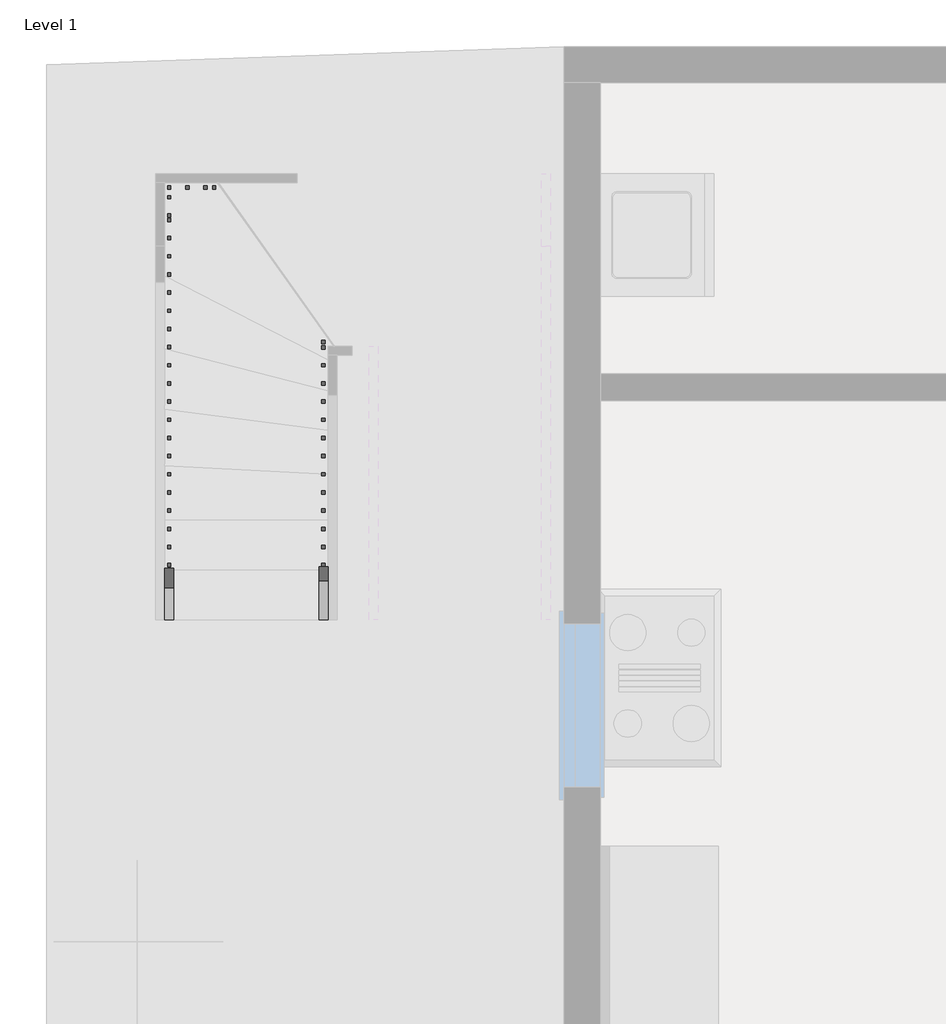
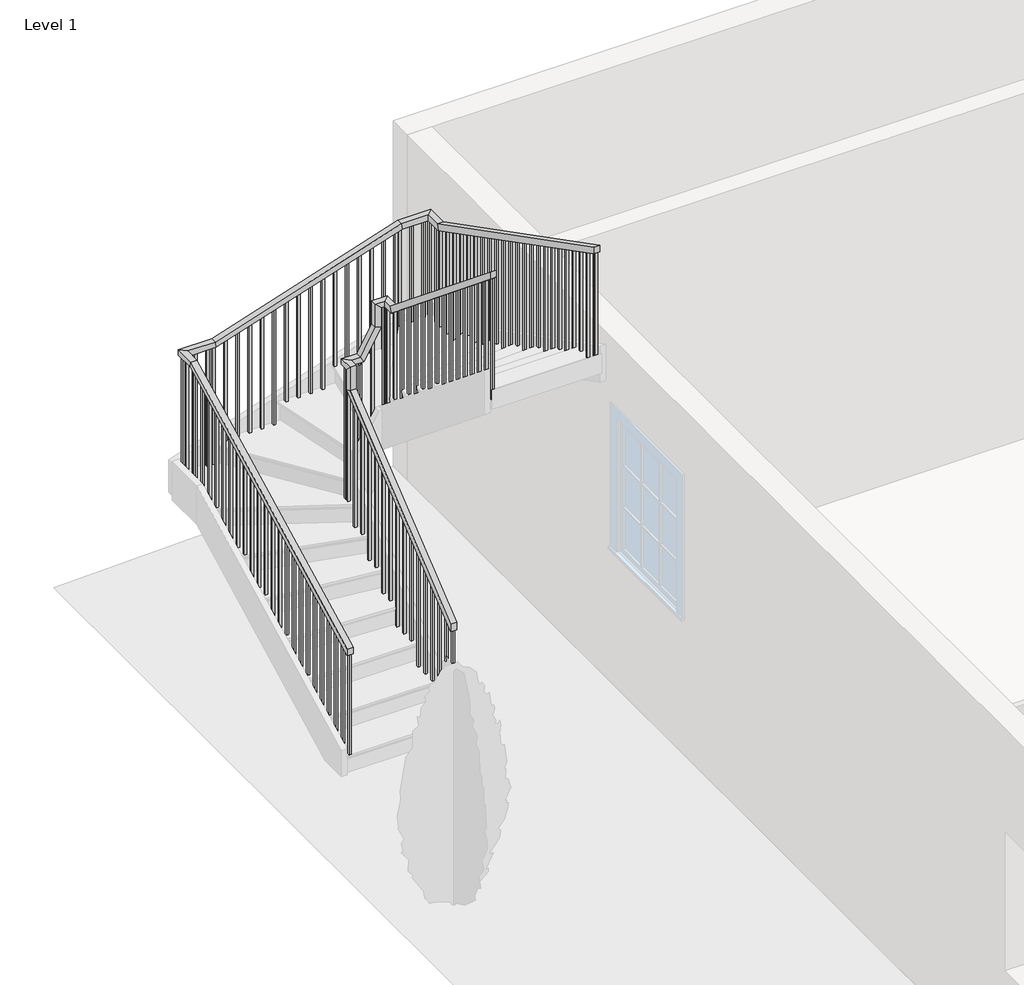
# One storey, part 2 of 3: 2 railings.
"""IFC4 building model written with IfcOpenShell, lengths in millimetres."""

from ifc_helpers import new_model, si_unit, frame, origin, place, context, project, spatial, polyline, outline, extrude, faceted_brep, element, save

model = new_model("IFC4")

# Units and contexts
model_context = context("Model", 3, world=origin())
ifc_project = project(units=[si_unit("LENGTHUNIT", "METRE", prefix="MILLI")], contexts=[model_context])

# Site, building, storey
site = spatial("IfcSite", under=ifc_project)
building = spatial("IfcBuilding", under=site)
storey = spatial("IfcBuildingStorey", under=building, Name="Level 1", Elevation=0.0)

# Railings
placement = place(None, origin())
element("IfcRailing", 1, ObjectType="Handrail - Rectangular", at=placement, inside=storey, context=model_context, shape_type="SolidModel", body=[
    faceted_brep([(-12458.9357228, 11608.7303252, 1025.2529681), (-12458.9357228, 11608.7303252, 959.7067088), (-12408.1357228, 11608.7303252, 959.7067088), (-12408.1357228, 11608.7303252, 1025.2529681), (-12458.9357228, 13060.2620171, 2208.7848338), (-12458.9357228, 13111.0620171, 2184.659247), (-12408.1357228, 13111.0620171, 2184.659247), (-12408.1357228, 13060.2620171, 2208.7848338), (-12458.9357228, 13060.2620171, 2414.6281882), (-12458.9357228, 13111.0620171, 2363.8281882), (-12408.1357228, 13111.0620171, 2363.8281882), (-12408.1357228, 13060.2620171, 2414.6281882), (-12458.9357228, 13187.2620171, 2414.6281882), (-12458.9357228, 13187.2620171, 2363.8281882), (-12408.1357228, 13136.4620171, 2363.8281882), (-12408.1357228, 13136.4620171, 2414.6281882), (-12331.9357228, 13187.2620171, 2414.6281882), (-12302.8143889, 13187.2620171, 2363.8281882), (-12302.8143889, 13136.4620171, 2363.8281882), (-12331.9357228, 13136.4620171, 2414.6281882), (-12204.9357228, 13187.2620171, 2631.5051451), (-12154.1357228, 13187.2620171, 2617.7256424), (-12154.1357228, 13136.4620171, 2617.7256424), (-12204.9357228, 13136.4620171, 2631.5051451), (-12204.9357228, 13187.2620171, 2837.3484995), (-12154.1357228, 13187.2620171, 2786.5484995), (-12154.1357228, 13136.4620171, 2786.5484995), (-12204.9357228, 13136.4620171, 2837.3484995), (-12077.9357228, 13187.2620171, 2837.3484995), (-12077.9357228, 13187.2620171, 2786.5484995), (-12128.7357228, 13136.4620171, 2786.5484995), (-12128.7357228, 13136.4620171, 2837.3484995), (-12077.9357228, 13060.2620171, 2837.3484995), (-12077.9357228, 13042.176604, 2786.5484995), (-12128.7357228, 13042.176604, 2786.5484995), (-12128.7357228, 13060.2620171, 2837.3484995), (-12077.9357228, 11608.7303252, 4020.8803652), (-12128.7357228, 11608.7303252, 4020.8803652), (-12128.7357228, 11608.7303252, 3955.3341059), (-12077.9357228, 11608.7303252, 3955.3341059)], [[[0, 1, 2, 3]], [[1, 0, 4, 5]], [[2, 1, 5, 6]], [[3, 2, 6, 7]], [[0, 3, 7, 4]], [[5, 4, 8, 9]], [[6, 5, 9, 10]], [[7, 6, 10, 11]], [[4, 7, 11, 8]], [[9, 8, 12, 13]], [[10, 9, 13, 14]], [[11, 10, 14, 15]], [[8, 11, 15, 12]], [[13, 12, 16, 17]], [[14, 13, 17, 18]], [[15, 14, 18, 19]], [[12, 15, 19, 16]], [[17, 16, 20, 21]], [[18, 17, 21, 22]], [[19, 18, 22, 23]], [[16, 19, 23, 20]], [[21, 20, 24, 25]], [[22, 21, 25, 26]], [[23, 22, 26, 27]], [[20, 23, 27, 24]], [[25, 24, 28, 29]], [[26, 25, 29, 30]], [[27, 26, 30, 31]], [[24, 27, 31, 28]], [[29, 28, 32, 33]], [[30, 29, 33, 34]], [[31, 30, 34, 35]], [[28, 31, 35, 32]], [[36, 37, 38, 39]], [[33, 32, 36, 39]], [[34, 33, 39, 38]], [[35, 34, 38, 37]], [[32, 35, 37, 36]]]),
    extrude(outline(polyline([(11698.9696608, 3881.7558784), (11718.0196608, 3866.2231262), (11718.0196608, 2878.6666667), (11698.9696608, 2878.6666667), (11698.9696608, 3881.7558784)])), frame((-12112.8607228, 0.0, 0.0), z_axis=(1.0, 0.0, 0.0), x_axis=(0.0, 1.0, 0.0)), (0.0, 0.0, 1.0), 19.05),
    extrude(outline(polyline([(11800.5696608, 3798.9145334), (11819.6196608, 3783.3817813), (11819.6196608, 2878.6666667), (11800.5696608, 2878.6666667), (11800.5696608, 3798.9145334)])), frame((-12112.8607228, 0.0, 0.0), z_axis=(1.0, 0.0, 0.0), x_axis=(0.0, 1.0, 0.0)), (0.0, 0.0, 1.0), 19.05),
    extrude(outline(polyline([(11902.1696608, 3716.0731885), (11921.2196608, 3700.5404364), (11921.2196608, 2709.3333333), (11902.1696608, 2709.3333333), (11902.1696608, 3716.0731885)])), frame((-12112.8607228, 0.0, 0.0), z_axis=(1.0, 0.0, 0.0), x_axis=(0.0, 1.0, 0.0)), (0.0, 0.0, 1.0), 19.05),
    extrude(outline(polyline([(12003.7696608, 3633.2318436), (12022.8196608, 3617.6990914), (12022.8196608, 2709.3333333), (12003.7696608, 2709.3333333), (12003.7696608, 3633.2318436)])), frame((-12112.8607228, 0.0, 0.0), z_axis=(1.0, 0.0, 0.0), x_axis=(0.0, 1.0, 0.0)), (0.0, 0.0, 1.0), 19.05),
    extrude(outline(polyline([(12105.3696608, 3550.3904987), (12124.4196608, 3534.8577465), (12124.4196608, 2709.3333333), (12105.3696608, 2709.3333333), (12105.3696608, 3550.3904987)])), frame((-12112.8607228, 0.0, 0.0), z_axis=(1.0, 0.0, 0.0), x_axis=(0.0, 1.0, 0.0)), (0.0, 0.0, 1.0), 19.05),
    extrude(outline(polyline([(12206.9696608, 3467.5491538), (12226.0196608, 3452.0164016), (12226.0196608, 2540.0), (12206.9696608, 2540.0), (12206.9696608, 3467.5491538)])), frame((-12112.8607228, 0.0, 0.0), z_axis=(1.0, 0.0, 0.0), x_axis=(0.0, 1.0, 0.0)), (0.0, 0.0, 1.0), 19.05),
    extrude(outline(polyline([(12308.5696608, 3384.7078088), (12327.6196608, 3369.1750567), (12327.6196608, 2540.0), (12308.5696608, 2540.0), (12308.5696608, 3384.7078088)])), frame((-12112.8607228, 0.0, 0.0), z_axis=(1.0, 0.0, 0.0), x_axis=(0.0, 1.0, 0.0)), (0.0, 0.0, 1.0), 19.05),
    extrude(outline(polyline([(12410.1696608, 3301.8664639), (12429.2196608, 3286.3337117), (12429.2196608, 2540.0), (12410.1696608, 2540.0), (12410.1696608, 3301.8664639)])), frame((-12112.8607228, 0.0, 0.0), z_axis=(1.0, 0.0, 0.0), x_axis=(0.0, 1.0, 0.0)), (0.0, 0.0, 1.0), 19.05),
    extrude(outline(polyline([(12511.7696608, 3219.025119), (12530.8196608, 3203.4923668), (12530.8196608, 2370.6666667), (12511.7696608, 2370.6666667), (12511.7696608, 3219.025119)])), frame((-12112.8607228, 0.0, 0.0), z_axis=(1.0, 0.0, 0.0), x_axis=(0.0, 1.0, 0.0)), (0.0, 0.0, 1.0), 19.05),
    extrude(outline(polyline([(12613.3696608, 3136.1837741), (12632.4196608, 3120.6510219), (12632.4196608, 2370.6666667), (12613.3696608, 2370.6666667), (12613.3696608, 3136.1837741)])), frame((-12112.8607228, 0.0, 0.0), z_axis=(1.0, 0.0, 0.0), x_axis=(0.0, 1.0, 0.0)), (0.0, 0.0, 1.0), 19.05),
    extrude(outline(polyline([(12714.9696608, 3053.3424291), (12734.0196608, 3037.809677), (12734.0196608, 2201.3333333), (12714.9696608, 2201.3333333), (12714.9696608, 3053.3424291)])), frame((-12112.8607228, 0.0, 0.0), z_axis=(1.0, 0.0, 0.0), x_axis=(0.0, 1.0, 0.0)), (0.0, 0.0, 1.0), 19.05),
    extrude(outline(polyline([(12816.5696608, 2970.5010842), (12835.6196608, 2954.9683321), (12835.6196608, 2201.3333333), (12816.5696608, 2201.3333333), (12816.5696608, 2970.5010842)])), frame((-12112.8607228, 0.0, 0.0), z_axis=(1.0, 0.0, 0.0), x_axis=(0.0, 1.0, 0.0)), (0.0, 0.0, 1.0), 19.05),
    extrude(outline(polyline([(12918.1696608, 2887.6597393), (12937.2196608, 2872.1269871), (12937.2196608, 2032.0), (12918.1696608, 2032.0), (12918.1696608, 2887.6597393)])), frame((-12112.8607228, 0.0, 0.0), z_axis=(1.0, 0.0, 0.0), x_axis=(0.0, 1.0, 0.0)), (0.0, 0.0, 1.0), 19.05),
    extrude(outline(polyline([(13019.7696608, 2804.8183944), (13038.8196608, 2789.2856422), (13038.8196608, 2032.0), (13019.7696608, 2032.0), (13019.7696608, 2804.8183944)])), frame((-12112.8607228, 0.0, 0.0), z_axis=(1.0, 0.0, 0.0), x_axis=(0.0, 1.0, 0.0)), (0.0, 0.0, 1.0), 19.05),
    extrude(outline(polyline([(2529.115018, -12206.024819), (2496.5834745, -12225.074819), (1524.0, -12225.074819), (1524.0, -12206.024819), (2529.115018, -12206.024819)])), frame((0.0, 13152.3370171, 0.0), z_axis=(0.0, 1.0, 0.0), x_axis=(0.0, 0.0, 1.0)), (0.0, 0.0, 1.0), 19.05),
    extrude(outline(polyline([(2355.6134525, -12307.624819), (2323.0819089, -12326.674819), (1524.0, -12326.674819), (1524.0, -12307.624819), (2355.6134525, -12307.624819)])), frame((0.0, 13152.3370171, 0.0), z_axis=(0.0, 1.0, 0.0), x_axis=(0.0, 0.0, 1.0)), (0.0, 0.0, 1.0), 19.05),
    extrude(outline(polyline([(13021.6053252, 2111.7191617), (13040.6553252, 2127.2519138), (13040.6553252, 1016.0), (13021.6053252, 1016.0), (13021.6053252, 2111.7191617)])), frame((-12443.0607228, 0.0, 0.0), z_axis=(1.0, 0.0, 0.0), x_axis=(0.0, 1.0, 0.0)), (0.0, 0.0, 1.0), 19.05),
    extrude(outline(polyline([(12920.0053252, 2028.8778167), (12939.0553252, 2044.4105689), (12939.0553252, 1016.0), (12920.0053252, 1016.0), (12920.0053252, 2028.8778167)])), frame((-12443.0607228, 0.0, 0.0), z_axis=(1.0, 0.0, 0.0), x_axis=(0.0, 1.0, 0.0)), (0.0, 0.0, 1.0), 19.05),
    extrude(outline(polyline([(12818.4053252, 1946.0364718), (12837.4553252, 1961.569224), (12837.4553252, 846.6666667), (12818.4053252, 846.6666667), (12818.4053252, 1946.0364718)])), frame((-12443.0607228, 0.0, 0.0), z_axis=(1.0, 0.0, 0.0), x_axis=(0.0, 1.0, 0.0)), (0.0, 0.0, 1.0), 19.05),
    extrude(outline(polyline([(12716.8053252, 1863.1951269), (12735.8553252, 1878.7278791), (12735.8553252, 846.6666667), (12716.8053252, 846.6666667), (12716.8053252, 1863.1951269)])), frame((-12443.0607228, 0.0, 0.0), z_axis=(1.0, 0.0, 0.0), x_axis=(0.0, 1.0, 0.0)), (0.0, 0.0, 1.0), 19.05),
    extrude(outline(polyline([(12615.2053252, 1780.353782), (12634.2553252, 1795.8865341), (12634.2553252, 677.3333333), (12615.2053252, 677.3333333), (12615.2053252, 1780.353782)])), frame((-12443.0607228, 0.0, 0.0), z_axis=(1.0, 0.0, 0.0), x_axis=(0.0, 1.0, 0.0)), (0.0, 0.0, 1.0), 19.05),
    extrude(outline(polyline([(12513.6053252, 1697.5124371), (12532.6553252, 1713.0451892), (12532.6553252, 677.3333333), (12513.6053252, 677.3333333), (12513.6053252, 1697.5124371)])), frame((-12443.0607228, 0.0, 0.0), z_axis=(1.0, 0.0, 0.0), x_axis=(0.0, 1.0, 0.0)), (0.0, 0.0, 1.0), 19.05),
    extrude(outline(polyline([(12412.0053252, 1614.6710921), (12431.0553252, 1630.2038443), (12431.0553252, 508.0), (12412.0053252, 508.0), (12412.0053252, 1614.6710921)])), frame((-12443.0607228, 0.0, 0.0), z_axis=(1.0, 0.0, 0.0), x_axis=(0.0, 1.0, 0.0)), (0.0, 0.0, 1.0), 19.05),
    extrude(outline(polyline([(12310.4053252, 1531.8297472), (12329.4553252, 1547.3624994), (12329.4553252, 508.0), (12310.4053252, 508.0), (12310.4053252, 1531.8297472)])), frame((-12443.0607228, 0.0, 0.0), z_axis=(1.0, 0.0, 0.0), x_axis=(0.0, 1.0, 0.0)), (0.0, 0.0, 1.0), 19.05),
    extrude(outline(polyline([(12208.8053252, 1448.9884023), (12227.8553252, 1464.5211545), (12227.8553252, 508.0), (12208.8053252, 508.0), (12208.8053252, 1448.9884023)])), frame((-12443.0607228, 0.0, 0.0), z_axis=(1.0, 0.0, 0.0), x_axis=(0.0, 1.0, 0.0)), (0.0, 0.0, 1.0), 19.05),
    extrude(outline(polyline([(12107.2053252, 1366.1470574), (12126.2553252, 1381.6798095), (12126.2553252, 338.6666667), (12107.2053252, 338.6666667), (12107.2053252, 1366.1470574)])), frame((-12443.0607228, 0.0, 0.0), z_axis=(1.0, 0.0, 0.0), x_axis=(0.0, 1.0, 0.0)), (0.0, 0.0, 1.0), 19.05),
    extrude(outline(polyline([(12005.6053252, 1283.3057124), (12024.6553252, 1298.8384646), (12024.6553252, 338.6666667), (12005.6053252, 338.6666667), (12005.6053252, 1283.3057124)])), frame((-12443.0607228, 0.0, 0.0), z_axis=(1.0, 0.0, 0.0), x_axis=(0.0, 1.0, 0.0)), (0.0, 0.0, 1.0), 19.05),
    extrude(outline(polyline([(11904.0053252, 1200.4643675), (11923.0553252, 1215.9971197), (11923.0553252, 338.6666667), (11904.0053252, 338.6666667), (11904.0053252, 1200.4643675)])), frame((-12443.0607228, 0.0, 0.0), z_axis=(1.0, 0.0, 0.0), x_axis=(0.0, 1.0, 0.0)), (0.0, 0.0, 1.0), 19.05),
    extrude(outline(polyline([(11802.4053252, 1117.6230226), (11821.4553252, 1133.1557748), (11821.4553252, 169.3333333), (11802.4053252, 169.3333333), (11802.4053252, 1117.6230226)])), frame((-12443.0607228, 0.0, 0.0), z_axis=(1.0, 0.0, 0.0), x_axis=(0.0, 1.0, 0.0)), (0.0, 0.0, 1.0), 19.05),
    extrude(outline(polyline([(11700.8053252, 1034.7816777), (11719.8553252, 1050.3144298), (11719.8553252, 169.3333333), (11700.8053252, 169.3333333), (11700.8053252, 1034.7816777)])), frame((-12443.0607228, 0.0, 0.0), z_axis=(1.0, 0.0, 0.0), x_axis=(0.0, 1.0, 0.0)), (0.0, 0.0, 1.0), 19.05),
    extrude(outline(polyline([(-12112.8607228, 13140.4196608), (-12093.8107228, 13140.4196608), (-12093.8107228, 13121.3696608), (-12112.8607228, 13121.3696608), (-12112.8607228, 13140.4196608)])), frame((0.0, 0.0, 1862.6666667), z_axis=(0.0, 0.0, 1.0), x_axis=(1.0, 0.0, 0.0)), (0.0, 0.0, 1.0), 923.8818329),
    extrude(outline(polyline([(-12112.8607228, 13152.3370171), (-12112.8607228, 13171.3870171), (-12093.8107228, 13171.3870171), (-12093.8107228, 13152.3370171), (-12112.8607228, 13152.3370171)])), frame((0.0, 0.0, 1862.6666667), z_axis=(0.0, 0.0, 1.0), x_axis=(1.0, 0.0, 0.0)), (0.0, 0.0, 1.0), 923.8818329),
    extrude(outline(polyline([(-12127.6466265, 13152.3370171), (-12127.6466265, 13171.3870171), (-12108.5966265, 13171.3870171), (-12108.5966265, 13152.3370171), (-12127.6466265, 13152.3370171)])), frame((0.0, 0.0, 1693.3333333), z_axis=(0.0, 0.0, 1.0), x_axis=(1.0, 0.0, 0.0)), (0.0, 0.0, 1.0), 1093.2151662),
    extrude(outline(polyline([(-12428.274819, 13152.3370171), (-12428.274819, 13171.3870171), (-12409.224819, 13171.3870171), (-12409.224819, 13152.3370171), (-12428.274819, 13152.3370171)])), frame((0.0, 0.0, 1354.6666667), z_axis=(0.0, 0.0, 1.0), x_axis=(1.0, 0.0, 0.0)), (0.0, 0.0, 1.0), 1009.1615215),
    extrude(outline(polyline([(-12424.0107228, 13152.3370171), (-12443.0607228, 13152.3370171), (-12443.0607228, 13171.3870171), (-12424.0107228, 13171.3870171), (-12424.0107228, 13152.3370171)])), frame((0.0, 0.0, 1185.3333333), z_axis=(0.0, 0.0, 1.0), x_axis=(1.0, 0.0, 0.0)), (0.0, 0.0, 1.0), 1178.4948549),
    extrude(outline(polyline([(-12424.0107228, 13121.3696608), (-12443.0607228, 13121.3696608), (-12443.0607228, 13140.4196608), (-12424.0107228, 13140.4196608), (-12424.0107228, 13121.3696608)])), frame((0.0, 0.0, 1185.3333333), z_axis=(0.0, 0.0, 1.0), x_axis=(1.0, 0.0, 0.0)), (0.0, 0.0, 1.0), 1178.4948549),
    extrude(outline(polyline([(11608.7303252, 3955.3341059), (11627.7803252, 3939.8013537), (11627.7803252, 2878.6666667), (11608.7303252, 2878.6666667), (11608.7303252, 3955.3341059)])), frame((-12112.8607228, 0.0, 0.0), z_axis=(1.0, 0.0, 0.0), x_axis=(0.0, 1.0, 0.0)), (0.0, 0.0, 1.0), 19.05),
    extrude(outline(polyline([(11608.7303252, 959.7067088), (11627.7803252, 975.239461), (11627.7803252, 169.3333333), (11608.7303252, 169.3333333), (11608.7303252, 959.7067088)])), frame((-12443.0607228, 0.0, 0.0), z_axis=(1.0, 0.0, 0.0), x_axis=(0.0, 1.0, 0.0)), (0.0, 0.0, 1.0), 19.05),
])
element("IfcRailing", 2, ObjectType="Handrail - Rectangular", at=placement, inside=storey, context=model_context, shape_type="SolidModel", body=[
    faceted_brep([(-13322.5357228, 11608.7303252, 1109.0771751), (-13322.5357228, 11608.7303252, 1051.9280057), (-13271.7357228, 11608.7303252, 1051.9280057), (-13271.7357228, 11608.7303252, 1109.0771751), (-13322.5357228, 13868.7121817, 2273.7644996), (-13322.5357228, 13881.032233, 2222.9644996), (-13271.7357228, 13881.032233, 2222.9644996), (-13271.7357228, 13868.7121817, 2273.7644996), (-13322.5357228, 14050.8620171, 2273.7644996), (-13322.5357228, 14050.8620171, 2222.9644996), (-13271.7357228, 14000.0620171, 2222.9644996), (-13271.7357228, 14000.0620171, 2273.7644996), (-13045.3817702, 14050.8620171, 2273.7644996), (-13037.431194, 14050.8620171, 2222.9644996), (-13037.431194, 14000.0620171, 2222.9644996), (-13045.3817702, 14000.0620171, 2273.7644996), (-11491.4896754, 14050.8620171, 2772.3688337), (-11483.5390993, 14050.8620171, 2721.5688337), (-11483.5390993, 14000.0620171, 2721.5688337), (-11491.4896754, 14000.0620171, 2772.3688337), (-11214.3357228, 14050.8620171, 2772.3688337), (-11214.3357228, 14050.8620171, 2721.5688337), (-11265.1357228, 14000.0620171, 2721.5688337), (-11265.1357228, 14000.0620171, 2772.3688337), (-11214.3357228, 13868.7121817, 2772.3688337), (-11214.3357228, 13856.3921304, 2721.5688337), (-11265.1357228, 13856.3921304, 2721.5688337), (-11265.1357228, 13868.7121817, 2772.3688337), (-11214.3357228, 11608.7303252, 3937.0561582), (-11265.1357228, 11608.7303252, 3937.0561582), (-11265.1357228, 11608.7303252, 3879.9069889), (-11214.3357228, 11608.7303252, 3879.9069889)], [[[0, 1, 2, 3]], [[1, 0, 4, 5]], [[2, 1, 5, 6]], [[3, 2, 6, 7]], [[0, 3, 7, 4]], [[5, 4, 8, 9]], [[6, 5, 9, 10]], [[7, 6, 10, 11]], [[4, 7, 11, 8]], [[9, 8, 12, 13]], [[10, 9, 13, 14]], [[11, 10, 14, 15]], [[8, 11, 15, 12]], [[13, 12, 16, 17]], [[14, 13, 17, 18]], [[15, 14, 18, 19]], [[12, 15, 19, 16]], [[17, 16, 20, 21]], [[18, 17, 21, 22]], [[19, 18, 22, 23]], [[16, 19, 23, 20]], [[21, 20, 24, 25]], [[22, 21, 25, 26]], [[23, 22, 26, 27]], [[20, 23, 27, 24]], [[28, 29, 30, 31]], [[25, 24, 28, 31]], [[26, 25, 31, 30]], [[27, 26, 30, 29]], [[24, 27, 29, 28]]]),
    extrude(outline(polyline([(11643.0371817, 3862.2268642), (11643.0371817, 2878.6666667), (11623.9871817, 2878.6666667), (11623.9871817, 3872.0443296), (11643.0371817, 3862.2268642)])), frame((-11249.2607228, 0.0, 0.0), z_axis=(1.0, 0.0, 0.0), x_axis=(0.0, 1.0, 0.0)), (0.0, 0.0, 1.0), 19.05),
    extrude(outline(polyline([(11744.6371817, 3809.8670491), (11744.6371817, 2878.6666667), (11725.5871817, 2878.6666667), (11725.5871817, 3819.6845145), (11744.6371817, 3809.8670491)])), frame((-11249.2607228, 0.0, 0.0), z_axis=(1.0, 0.0, 0.0), x_axis=(0.0, 1.0, 0.0)), (0.0, 0.0, 1.0), 19.05),
    extrude(outline(polyline([(11846.2371817, 3757.507234), (11846.2371817, 2878.6666667), (11827.1871817, 2878.6666667), (11827.1871817, 3767.3246993), (11846.2371817, 3757.507234)])), frame((-11249.2607228, 0.0, 0.0), z_axis=(1.0, 0.0, 0.0), x_axis=(0.0, 1.0, 0.0)), (0.0, 0.0, 1.0), 19.05),
    extrude(outline(polyline([(11947.8371817, 3705.1474189), (11947.8371817, 2709.3333333), (11928.7871817, 2709.3333333), (11928.7871817, 3714.9648842), (11947.8371817, 3705.1474189)])), frame((-11249.2607228, 0.0, 0.0), z_axis=(1.0, 0.0, 0.0), x_axis=(0.0, 1.0, 0.0)), (0.0, 0.0, 1.0), 19.05),
    extrude(outline(polyline([(12049.4371817, 3652.7876038), (12049.4371817, 2709.3333333), (12030.3871817, 2709.3333333), (12030.3871817, 3662.6050691), (12049.4371817, 3652.7876038)])), frame((-11249.2607228, 0.0, 0.0), z_axis=(1.0, 0.0, 0.0), x_axis=(0.0, 1.0, 0.0)), (0.0, 0.0, 1.0), 19.05),
    extrude(outline(polyline([(12151.0371817, 3600.4277887), (12151.0371817, 2709.3333333), (12131.9871817, 2709.3333333), (12131.9871817, 3610.245254), (12151.0371817, 3600.4277887)])), frame((-11249.2607228, 0.0, 0.0), z_axis=(1.0, 0.0, 0.0), x_axis=(0.0, 1.0, 0.0)), (0.0, 0.0, 1.0), 19.05),
    extrude(outline(polyline([(12252.6371817, 3548.0679735), (12252.6371817, 2540.0), (12233.5871817, 2540.0), (12233.5871817, 3557.8854389), (12252.6371817, 3548.0679735)])), frame((-11249.2607228, 0.0, 0.0), z_axis=(1.0, 0.0, 0.0), x_axis=(0.0, 1.0, 0.0)), (0.0, 0.0, 1.0), 19.05),
    extrude(outline(polyline([(12354.2371817, 3495.7081584), (12354.2371817, 2540.0), (12335.1871817, 2540.0), (12335.1871817, 3505.5256238), (12354.2371817, 3495.7081584)])), frame((-11249.2607228, 0.0, 0.0), z_axis=(1.0, 0.0, 0.0), x_axis=(0.0, 1.0, 0.0)), (0.0, 0.0, 1.0), 19.05),
    extrude(outline(polyline([(12455.8371817, 3443.3483433), (12455.8371817, 2540.0), (12436.7871817, 2540.0), (12436.7871817, 3453.1658086), (12455.8371817, 3443.3483433)])), frame((-11249.2607228, 0.0, 0.0), z_axis=(1.0, 0.0, 0.0), x_axis=(0.0, 1.0, 0.0)), (0.0, 0.0, 1.0), 19.05),
    extrude(outline(polyline([(12557.4371817, 3390.9885282), (12557.4371817, 2370.6666667), (12538.3871817, 2370.6666667), (12538.3871817, 3400.8059935), (12557.4371817, 3390.9885282)])), frame((-11249.2607228, 0.0, 0.0), z_axis=(1.0, 0.0, 0.0), x_axis=(0.0, 1.0, 0.0)), (0.0, 0.0, 1.0), 19.05),
    extrude(outline(polyline([(12659.0371817, 3338.6287131), (12659.0371817, 2370.6666667), (12639.9871817, 2370.6666667), (12639.9871817, 3348.4461784), (12659.0371817, 3338.6287131)])), frame((-11249.2607228, 0.0, 0.0), z_axis=(1.0, 0.0, 0.0), x_axis=(0.0, 1.0, 0.0)), (0.0, 0.0, 1.0), 19.05),
    extrude(outline(polyline([(12760.6371817, 3286.268898), (12760.6371817, 2370.6666667), (12741.5871817, 2370.6666667), (12741.5871817, 3296.0863633), (12760.6371817, 3286.268898)])), frame((-11249.2607228, 0.0, 0.0), z_axis=(1.0, 0.0, 0.0), x_axis=(0.0, 1.0, 0.0)), (0.0, 0.0, 1.0), 19.05),
    extrude(outline(polyline([(12862.2371817, 3233.9090828), (12862.2371817, 2201.3333333), (12843.1871817, 2201.3333333), (12843.1871817, 3243.7265482), (12862.2371817, 3233.9090828)])), frame((-11249.2607228, 0.0, 0.0), z_axis=(1.0, 0.0, 0.0), x_axis=(0.0, 1.0, 0.0)), (0.0, 0.0, 1.0), 19.05),
    extrude(outline(polyline([(12963.8371817, 3181.5492677), (12963.8371817, 2201.3333333), (12944.7871817, 2201.3333333), (12944.7871817, 3191.3667331), (12963.8371817, 3181.5492677)])), frame((-11249.2607228, 0.0, 0.0), z_axis=(1.0, 0.0, 0.0), x_axis=(0.0, 1.0, 0.0)), (0.0, 0.0, 1.0), 19.05),
    extrude(outline(polyline([(13065.4371817, 3129.1894526), (13065.4371817, 2201.3333333), (13046.3871817, 2201.3333333), (13046.3871817, 3139.0069179), (13065.4371817, 3129.1894526)])), frame((-11249.2607228, 0.0, 0.0), z_axis=(1.0, 0.0, 0.0), x_axis=(0.0, 1.0, 0.0)), (0.0, 0.0, 1.0), 19.05),
    extrude(outline(polyline([(13167.0371817, 3076.8296375), (13167.0371817, 2032.0), (13147.9871817, 2032.0), (13147.9871817, 3086.6471028), (13167.0371817, 3076.8296375)])), frame((-11249.2607228, 0.0, 0.0), z_axis=(1.0, 0.0, 0.0), x_axis=(0.0, 1.0, 0.0)), (0.0, 0.0, 1.0), 19.05),
    extrude(outline(polyline([(13268.6371817, 3024.4698224), (13268.6371817, 2032.0), (13249.5871817, 2032.0), (13249.5871817, 3034.2872877), (13268.6371817, 3024.4698224)])), frame((-11249.2607228, 0.0, 0.0), z_axis=(1.0, 0.0, 0.0), x_axis=(0.0, 1.0, 0.0)), (0.0, 0.0, 1.0), 19.05),
    extrude(outline(polyline([(13370.2371817, 2972.1100073), (13370.2371817, 2032.0), (13351.1871817, 2032.0), (13351.1871817, 2981.9274726), (13370.2371817, 2972.1100073)])), frame((-11249.2607228, 0.0, 0.0), z_axis=(1.0, 0.0, 0.0), x_axis=(0.0, 1.0, 0.0)), (0.0, 0.0, 1.0), 19.05),
    extrude(outline(polyline([(13471.8371817, 2919.7501921), (13471.8371817, 2032.0), (13452.7871817, 2032.0), (13452.7871817, 2929.5676575), (13471.8371817, 2919.7501921)])), frame((-11249.2607228, 0.0, 0.0), z_axis=(1.0, 0.0, 0.0), x_axis=(0.0, 1.0, 0.0)), (0.0, 0.0, 1.0), 19.05),
    extrude(outline(polyline([(13573.4371817, 2867.390377), (13573.4371817, 1862.6666667), (13554.3871817, 1862.6666667), (13554.3871817, 2877.2078424), (13573.4371817, 2867.390377)])), frame((-11249.2607228, 0.0, 0.0), z_axis=(1.0, 0.0, 0.0), x_axis=(0.0, 1.0, 0.0)), (0.0, 0.0, 1.0), 19.05),
    extrude(outline(polyline([(13675.0371817, 2815.0305619), (13675.0371817, 1862.6666667), (13655.9871817, 1862.6666667), (13655.9871817, 2824.8480272), (13675.0371817, 2815.0305619)])), frame((-11249.2607228, 0.0, 0.0), z_axis=(1.0, 0.0, 0.0), x_axis=(0.0, 1.0, 0.0)), (0.0, 0.0, 1.0), 19.05),
    extrude(outline(polyline([(13776.6371817, 2762.6707468), (13776.6371817, 1862.6666667), (13757.5871817, 1862.6666667), (13757.5871817, 2772.4882121), (13776.6371817, 2762.6707468)])), frame((-11249.2607228, 0.0, 0.0), z_axis=(1.0, 0.0, 0.0), x_axis=(0.0, 1.0, 0.0)), (0.0, 0.0, 1.0), 19.05),
    extrude(outline(polyline([(-11230.2107228, 13933.3870171), (-11230.2107228, 13914.3370171), (-11249.2607228, 13914.3370171), (-11249.2607228, 13933.3870171), (-11230.2107228, 13933.3870171)])), frame((0.0, 0.0, 1862.6666667), z_axis=(0.0, 0.0, 1.0), x_axis=(1.0, 0.0, 0.0)), (0.0, 0.0, 1.0), 858.902167),
    extrude(outline(polyline([(-11297.8146754, 14034.9870171), (-11278.7646754, 14034.9870171), (-11278.7646754, 14015.9370171), (-11297.8146754, 14015.9370171), (-11297.8146754, 14034.9870171)])), frame((0.0, 0.0, 1862.6666667), z_axis=(0.0, 0.0, 1.0), x_axis=(1.0, 0.0, 0.0)), (0.0, 0.0, 1.0), 858.902167),
    extrude(outline(polyline([(-11399.4146754, 14034.9870171), (-11380.3646754, 14034.9870171), (-11380.3646754, 14015.9370171), (-11399.4146754, 14015.9370171), (-11399.4146754, 14034.9870171)])), frame((0.0, 0.0, 1862.6666667), z_axis=(0.0, 0.0, 1.0), x_axis=(1.0, 0.0, 0.0)), (0.0, 0.0, 1.0), 858.902167),
    extrude(outline(polyline([(2706.3697564, -11530.9067702), (1693.3333333, -11530.9067702), (1693.3333333, -11511.8567702), (2712.4824155, -11511.8567702), (2706.3697564, -11530.9067702)])), frame((0.0, 14015.9370171, 0.0), z_axis=(0.0, 1.0, 0.0), x_axis=(0.0, 0.0, 1.0)), (0.0, 0.0, 1.0), 19.05),
    extrude(outline(polyline([(2673.7689082, -11632.5067702), (1693.3333333, -11632.5067702), (1693.3333333, -11613.4567702), (2679.8815673, -11613.4567702), (2673.7689082, -11632.5067702)])), frame((0.0, 14015.9370171, 0.0), z_axis=(0.0, 1.0, 0.0), x_axis=(0.0, 0.0, 1.0)), (0.0, 0.0, 1.0), 19.05),
    extrude(outline(polyline([(2641.16806, -11734.1067702), (1693.3333333, -11734.1067702), (1693.3333333, -11715.0567702), (2647.280719, -11715.0567702), (2641.16806, -11734.1067702)])), frame((0.0, 14015.9370171, 0.0), z_axis=(0.0, 1.0, 0.0), x_axis=(0.0, 0.0, 1.0)), (0.0, 0.0, 1.0), 19.05),
    extrude(outline(polyline([(2608.5672118, -11835.7067702), (1693.3333333, -11835.7067702), (1693.3333333, -11816.6567702), (2614.6798708, -11816.6567702), (2608.5672118, -11835.7067702)])), frame((0.0, 14015.9370171, 0.0), z_axis=(0.0, 1.0, 0.0), x_axis=(0.0, 0.0, 1.0)), (0.0, 0.0, 1.0), 19.05),
    extrude(outline(polyline([(2575.9663635, -11937.3067702), (1693.3333333, -11937.3067702), (1693.3333333, -11918.2567702), (2582.0790226, -11918.2567702), (2575.9663635, -11937.3067702)])), frame((0.0, 14015.9370171, 0.0), z_axis=(0.0, 1.0, 0.0), x_axis=(0.0, 0.0, 1.0)), (0.0, 0.0, 1.0), 19.05),
    extrude(outline(polyline([(2543.3655153, -12038.9067702), (1693.3333333, -12038.9067702), (1693.3333333, -12019.8567702), (2549.4781744, -12019.8567702), (2543.3655153, -12038.9067702)])), frame((0.0, 14015.9370171, 0.0), z_axis=(0.0, 1.0, 0.0), x_axis=(0.0, 0.0, 1.0)), (0.0, 0.0, 1.0), 19.05),
    extrude(outline(polyline([(2510.7646671, -12140.5067702), (1524.0, -12140.5067702), (1524.0, -12121.4567702), (2516.8773261, -12121.4567702), (2510.7646671, -12140.5067702)])), frame((0.0, 14015.9370171, 0.0), z_axis=(0.0, 1.0, 0.0), x_axis=(0.0, 0.0, 1.0)), (0.0, 0.0, 1.0), 19.05),
    extrude(outline(polyline([(2478.1638189, -12242.1067702), (1524.0, -12242.1067702), (1524.0, -12223.0567702), (2484.2764779, -12223.0567702), (2478.1638189, -12242.1067702)])), frame((0.0, 14015.9370171, 0.0), z_axis=(0.0, 1.0, 0.0), x_axis=(0.0, 0.0, 1.0)), (0.0, 0.0, 1.0), 19.05),
    extrude(outline(polyline([(2445.5629706, -12343.7067702), (1524.0, -12343.7067702), (1524.0, -12324.6567702), (2451.6756297, -12324.6567702), (2445.5629706, -12343.7067702)])), frame((0.0, 14015.9370171, 0.0), z_axis=(0.0, 1.0, 0.0), x_axis=(0.0, 0.0, 1.0)), (0.0, 0.0, 1.0), 19.05),
    extrude(outline(polyline([(2412.9621224, -12445.3067702), (1524.0, -12445.3067702), (1524.0, -12426.2567702), (2419.0747814, -12426.2567702), (2412.9621224, -12445.3067702)])), frame((0.0, 14015.9370171, 0.0), z_axis=(0.0, 1.0, 0.0), x_axis=(0.0, 0.0, 1.0)), (0.0, 0.0, 1.0), 19.05),
    extrude(outline(polyline([(2380.3612742, -12546.9067702), (1354.6666667, -12546.9067702), (1354.6666667, -12527.8567702), (2386.4739332, -12527.8567702), (2380.3612742, -12546.9067702)])), frame((0.0, 14015.9370171, 0.0), z_axis=(0.0, 1.0, 0.0), x_axis=(0.0, 0.0, 1.0)), (0.0, 0.0, 1.0), 19.05),
    extrude(outline(polyline([(2347.7604259, -12648.5067702), (1354.6666667, -12648.5067702), (1354.6666667, -12629.4567702), (2353.873085, -12629.4567702), (2347.7604259, -12648.5067702)])), frame((0.0, 14015.9370171, 0.0), z_axis=(0.0, 1.0, 0.0), x_axis=(0.0, 0.0, 1.0)), (0.0, 0.0, 1.0), 19.05),
    extrude(outline(polyline([(2315.1595777, -12750.1067702), (1354.6666667, -12750.1067702), (1354.6666667, -12731.0567702), (2321.2722368, -12731.0567702), (2315.1595777, -12750.1067702)])), frame((0.0, 14015.9370171, 0.0), z_axis=(0.0, 1.0, 0.0), x_axis=(0.0, 0.0, 1.0)), (0.0, 0.0, 1.0), 19.05),
    extrude(outline(polyline([(2282.5587295, -12851.7067702), (1354.6666667, -12851.7067702), (1354.6666667, -12832.6567702), (2288.6713885, -12832.6567702), (2282.5587295, -12851.7067702)])), frame((0.0, 14015.9370171, 0.0), z_axis=(0.0, 1.0, 0.0), x_axis=(0.0, 0.0, 1.0)), (0.0, 0.0, 1.0), 19.05),
    extrude(outline(polyline([(2249.9578813, -12953.3067702), (1354.6666667, -12953.3067702), (1354.6666667, -12934.2567702), (2256.0705403, -12934.2567702), (2249.9578813, -12953.3067702)])), frame((0.0, 14015.9370171, 0.0), z_axis=(0.0, 1.0, 0.0), x_axis=(0.0, 0.0, 1.0)), (0.0, 0.0, 1.0), 19.05),
    extrude(outline(polyline([(-13103.4607228, 14034.9870171), (-13084.4107228, 14034.9870171), (-13084.4107228, 14015.9370171), (-13103.4607228, 14015.9370171), (-13103.4607228, 14034.9870171)])), frame((0.0, 0.0, 1185.3333333), z_axis=(0.0, 0.0, 1.0), x_axis=(1.0, 0.0, 0.0)), (0.0, 0.0, 1.0), 1037.6311663),
    extrude(outline(polyline([(-13205.0607228, 14034.9870171), (-13186.0107228, 14034.9870171), (-13186.0107228, 14015.9370171), (-13205.0607228, 14015.9370171), (-13205.0607228, 14034.9870171)])), frame((0.0, 0.0, 1185.3333333), z_axis=(0.0, 0.0, 1.0), x_axis=(1.0, 0.0, 0.0)), (0.0, 0.0, 1.0), 1037.6311663),
    extrude(outline(polyline([(-13306.6607228, 13960.7871817), (-13306.6607228, 13979.8371817), (-13287.6107228, 13979.8371817), (-13287.6107228, 13960.7871817), (-13306.6607228, 13960.7871817)])), frame((0.0, 0.0, 1185.3333333), z_axis=(0.0, 0.0, 1.0), x_axis=(1.0, 0.0, 0.0)), (0.0, 0.0, 1.0), 1037.6311663),
    extrude(outline(polyline([(13853.4553252, 2208.752671), (13853.4553252, 1185.3333333), (13834.4053252, 1185.3333333), (13834.4053252, 2198.9352056), (13853.4553252, 2208.752671)])), frame((-13306.6607228, 0.0, 0.0), z_axis=(1.0, 0.0, 0.0), x_axis=(0.0, 1.0, 0.0)), (0.0, 0.0, 1.0), 19.05),
    extrude(outline(polyline([(13751.8553252, 2156.3928558), (13751.8553252, 1185.3333333), (13732.8053252, 1185.3333333), (13732.8053252, 2146.5753905), (13751.8553252, 2156.3928558)])), frame((-13306.6607228, 0.0, 0.0), z_axis=(1.0, 0.0, 0.0), x_axis=(0.0, 1.0, 0.0)), (0.0, 0.0, 1.0), 19.05),
    extrude(outline(polyline([(13650.2553252, 2104.0330407), (13650.2553252, 1185.3333333), (13631.2053252, 1185.3333333), (13631.2053252, 2094.2155754), (13650.2553252, 2104.0330407)])), frame((-13306.6607228, 0.0, 0.0), z_axis=(1.0, 0.0, 0.0), x_axis=(0.0, 1.0, 0.0)), (0.0, 0.0, 1.0), 19.05),
    extrude(outline(polyline([(13548.6553252, 2051.6732256), (13548.6553252, 1185.3333333), (13529.6053252, 1185.3333333), (13529.6053252, 2041.8557603), (13548.6553252, 2051.6732256)])), frame((-13306.6607228, 0.0, 0.0), z_axis=(1.0, 0.0, 0.0), x_axis=(0.0, 1.0, 0.0)), (0.0, 0.0, 1.0), 19.05),
    extrude(outline(polyline([(13447.0553252, 1999.3134105), (13447.0553252, 1016.0), (13428.0053252, 1016.0), (13428.0053252, 1989.4959452), (13447.0553252, 1999.3134105)])), frame((-13306.6607228, 0.0, 0.0), z_axis=(1.0, 0.0, 0.0), x_axis=(0.0, 1.0, 0.0)), (0.0, 0.0, 1.0), 19.05),
    extrude(outline(polyline([(13345.4553252, 1946.9535954), (13345.4553252, 1016.0), (13326.4053252, 1016.0), (13326.4053252, 1937.13613), (13345.4553252, 1946.9535954)])), frame((-13306.6607228, 0.0, 0.0), z_axis=(1.0, 0.0, 0.0), x_axis=(0.0, 1.0, 0.0)), (0.0, 0.0, 1.0), 19.05),
    extrude(outline(polyline([(13243.8553252, 1894.5937803), (13243.8553252, 1016.0), (13224.8053252, 1016.0), (13224.8053252, 1884.7763149), (13243.8553252, 1894.5937803)])), frame((-13306.6607228, 0.0, 0.0), z_axis=(1.0, 0.0, 0.0), x_axis=(0.0, 1.0, 0.0)), (0.0, 0.0, 1.0), 19.05),
    extrude(outline(polyline([(13142.2553252, 1842.2339651), (13142.2553252, 1016.0), (13123.2053252, 1016.0), (13123.2053252, 1832.4164998), (13142.2553252, 1842.2339651)])), frame((-13306.6607228, 0.0, 0.0), z_axis=(1.0, 0.0, 0.0), x_axis=(0.0, 1.0, 0.0)), (0.0, 0.0, 1.0), 19.05),
    extrude(outline(polyline([(13040.6553252, 1789.87415), (13040.6553252, 846.6666667), (13021.6053252, 846.6666667), (13021.6053252, 1780.0566847), (13040.6553252, 1789.87415)])), frame((-13306.6607228, 0.0, 0.0), z_axis=(1.0, 0.0, 0.0), x_axis=(0.0, 1.0, 0.0)), (0.0, 0.0, 1.0), 19.05),
    extrude(outline(polyline([(12939.0553252, 1737.5143349), (12939.0553252, 846.6666667), (12920.0053252, 846.6666667), (12920.0053252, 1727.6968696), (12939.0553252, 1737.5143349)])), frame((-13306.6607228, 0.0, 0.0), z_axis=(1.0, 0.0, 0.0), x_axis=(0.0, 1.0, 0.0)), (0.0, 0.0, 1.0), 19.05),
    extrude(outline(polyline([(12837.4553252, 1685.1545198), (12837.4553252, 846.6666667), (12818.4053252, 846.6666667), (12818.4053252, 1675.3370545), (12837.4553252, 1685.1545198)])), frame((-13306.6607228, 0.0, 0.0), z_axis=(1.0, 0.0, 0.0), x_axis=(0.0, 1.0, 0.0)), (0.0, 0.0, 1.0), 19.05),
    extrude(outline(polyline([(12735.8553252, 1632.7947047), (12735.8553252, 677.3333333), (12716.8053252, 677.3333333), (12716.8053252, 1622.9772393), (12735.8553252, 1632.7947047)])), frame((-13306.6607228, 0.0, 0.0), z_axis=(1.0, 0.0, 0.0), x_axis=(0.0, 1.0, 0.0)), (0.0, 0.0, 1.0), 19.05),
    extrude(outline(polyline([(12634.2553252, 1580.4348896), (12634.2553252, 677.3333333), (12615.2053252, 677.3333333), (12615.2053252, 1570.6174242), (12634.2553252, 1580.4348896)])), frame((-13306.6607228, 0.0, 0.0), z_axis=(1.0, 0.0, 0.0), x_axis=(0.0, 1.0, 0.0)), (0.0, 0.0, 1.0), 19.05),
    extrude(outline(polyline([(12532.6553252, 1528.0750744), (12532.6553252, 677.3333333), (12513.6053252, 677.3333333), (12513.6053252, 1518.2576091), (12532.6553252, 1528.0750744)])), frame((-13306.6607228, 0.0, 0.0), z_axis=(1.0, 0.0, 0.0), x_axis=(0.0, 1.0, 0.0)), (0.0, 0.0, 1.0), 19.05),
    extrude(outline(polyline([(12431.0553252, 1475.7152593), (12431.0553252, 508.0), (12412.0053252, 508.0), (12412.0053252, 1465.897794), (12431.0553252, 1475.7152593)])), frame((-13306.6607228, 0.0, 0.0), z_axis=(1.0, 0.0, 0.0), x_axis=(0.0, 1.0, 0.0)), (0.0, 0.0, 1.0), 19.05),
    extrude(outline(polyline([(12329.4553252, 1423.3554442), (12329.4553252, 508.0), (12310.4053252, 508.0), (12310.4053252, 1413.5379789), (12329.4553252, 1423.3554442)])), frame((-13306.6607228, 0.0, 0.0), z_axis=(1.0, 0.0, 0.0), x_axis=(0.0, 1.0, 0.0)), (0.0, 0.0, 1.0), 19.05),
    extrude(outline(polyline([(12227.8553252, 1370.9956291), (12227.8553252, 508.0), (12208.8053252, 508.0), (12208.8053252, 1361.1781638), (12227.8553252, 1370.9956291)])), frame((-13306.6607228, 0.0, 0.0), z_axis=(1.0, 0.0, 0.0), x_axis=(0.0, 1.0, 0.0)), (0.0, 0.0, 1.0), 19.05),
    extrude(outline(polyline([(12126.2553252, 1318.635814), (12126.2553252, 338.6666667), (12107.2053252, 338.6666667), (12107.2053252, 1308.8183486), (12126.2553252, 1318.635814)])), frame((-13306.6607228, 0.0, 0.0), z_axis=(1.0, 0.0, 0.0), x_axis=(0.0, 1.0, 0.0)), (0.0, 0.0, 1.0), 19.05),
    extrude(outline(polyline([(12024.6553252, 1266.2759989), (12024.6553252, 338.6666667), (12005.6053252, 338.6666667), (12005.6053252, 1256.4585335), (12024.6553252, 1266.2759989)])), frame((-13306.6607228, 0.0, 0.0), z_axis=(1.0, 0.0, 0.0), x_axis=(0.0, 1.0, 0.0)), (0.0, 0.0, 1.0), 19.05),
    extrude(outline(polyline([(11923.0553252, 1213.9161837), (11923.0553252, 338.6666667), (11904.0053252, 338.6666667), (11904.0053252, 1204.0987184), (11923.0553252, 1213.9161837)])), frame((-13306.6607228, 0.0, 0.0), z_axis=(1.0, 0.0, 0.0), x_axis=(0.0, 1.0, 0.0)), (0.0, 0.0, 1.0), 19.05),
    extrude(outline(polyline([(11821.4553252, 1161.5563686), (11821.4553252, 169.3333333), (11802.4053252, 169.3333333), (11802.4053252, 1151.7389033), (11821.4553252, 1161.5563686)])), frame((-13306.6607228, 0.0, 0.0), z_axis=(1.0, 0.0, 0.0), x_axis=(0.0, 1.0, 0.0)), (0.0, 0.0, 1.0), 19.05),
    extrude(outline(polyline([(11719.8553252, 1109.1965535), (11719.8553252, 169.3333333), (11700.8053252, 169.3333333), (11700.8053252, 1099.3790882), (11719.8553252, 1109.1965535)])), frame((-13306.6607228, 0.0, 0.0), z_axis=(1.0, 0.0, 0.0), x_axis=(0.0, 1.0, 0.0)), (0.0, 0.0, 1.0), 19.05),
    extrude(outline(polyline([(-11230.2107228, 13878.2371817), (-11230.2107228, 13859.1871817), (-11249.2607228, 13859.1871817), (-11249.2607228, 13878.2371817), (-11230.2107228, 13878.2371817)])), frame((0.0, 0.0, 1862.6666667), z_axis=(0.0, 0.0, 1.0), x_axis=(1.0, 0.0, 0.0)), (0.0, 0.0, 1.0), 858.902167),
    extrude(outline(polyline([(-11249.2607228, 14034.9870171), (-11230.2107228, 14034.9870171), (-11230.2107228, 14015.9370171), (-11249.2607228, 14015.9370171), (-11249.2607228, 14034.9870171)])), frame((0.0, 0.0, 1862.6666667), z_axis=(0.0, 0.0, 1.0), x_axis=(1.0, 0.0, 0.0)), (0.0, 0.0, 1.0), 858.902167),
    extrude(outline(polyline([(2715.9613671, -11501.0146754), (1862.6666667, -11501.0146754), (1862.6666667, -11481.9646754), (2722.0740262, -11481.9646754), (2715.9613671, -11501.0146754)])), frame((0.0, 14015.9370171, 0.0), z_axis=(0.0, 1.0, 0.0), x_axis=(0.0, 0.0, 1.0)), (0.0, 0.0, 1.0), 19.05),
    extrude(outline(polyline([(-13054.9067702, 14034.9870171), (-13035.8567702, 14034.9870171), (-13035.8567702, 14015.9370171), (-13054.9067702, 14015.9370171), (-13054.9067702, 14034.9870171)])), frame((0.0, 0.0, 1185.3333333), z_axis=(0.0, 0.0, 1.0), x_axis=(1.0, 0.0, 0.0)), (0.0, 0.0, 1.0), 1037.6311663),
    extrude(outline(polyline([(-13306.6607228, 14015.9370171), (-13306.6607228, 14034.9870171), (-13287.6107228, 14034.9870171), (-13287.6107228, 14015.9370171), (-13306.6607228, 14015.9370171)])), frame((0.0, 0.0, 1185.3333333), z_axis=(0.0, 0.0, 1.0), x_axis=(1.0, 0.0, 0.0)), (0.0, 0.0, 1.0), 1037.6311663),
    extrude(outline(polyline([(13878.2371817, 2221.5240629), (13878.2371817, 1185.3333333), (13859.1871817, 1185.3333333), (13859.1871817, 2211.7065976), (13878.2371817, 2221.5240629)])), frame((-13306.6607228, 0.0, 0.0), z_axis=(1.0, 0.0, 0.0), x_axis=(0.0, 1.0, 0.0)), (0.0, 0.0, 1.0), 19.05),
    extrude(outline(polyline([(11627.7803252, 3870.0895235), (11627.7803252, 2878.6666667), (11608.7303252, 2878.6666667), (11608.7303252, 3879.9069889), (11627.7803252, 3870.0895235)])), frame((-11249.2607228, 0.0, 0.0), z_axis=(1.0, 0.0, 0.0), x_axis=(0.0, 1.0, 0.0)), (0.0, 0.0, 1.0), 19.05),
    extrude(outline(polyline([(11627.7803252, 1061.7454711), (11627.7803252, 169.3333333), (11608.7303252, 169.3333333), (11608.7303252, 1051.9280057), (11627.7803252, 1061.7454711)])), frame((-13306.6607228, 0.0, 0.0), z_axis=(1.0, 0.0, 0.0), x_axis=(0.0, 1.0, 0.0)), (0.0, 0.0, 1.0), 19.05),
])

save(model, "model.ifc")

# Revit data of these elements
# Type "Handrail - Rectangular"
#   Assembly Code = "C2010400"
#   built-in parameter 1008612 = 0.0416667 (stored number, unit not read)
#   built-in parameter 1008611 = 0.0416667 (stored number, unit not read)
#   built-in parameter 1008609 = 0.333333 (stored number, unit not read)
#   built-in parameter 1008604 = 0.166667 (stored number, unit not read)
#   built-in parameter 1008603 = 0.166667 (stored number, unit not read)
#   Railing Height = 3' - 0"
#   built-in parameter 1008630 = 2
#   built-in parameter 1008610 = 2
#   built-in parameter 1008618 = Baluster - Square : 3/4"
# Elements 1, 2 (IfcRailing, "Handrail - Rectangular")
#   Phase Created = New Construction
